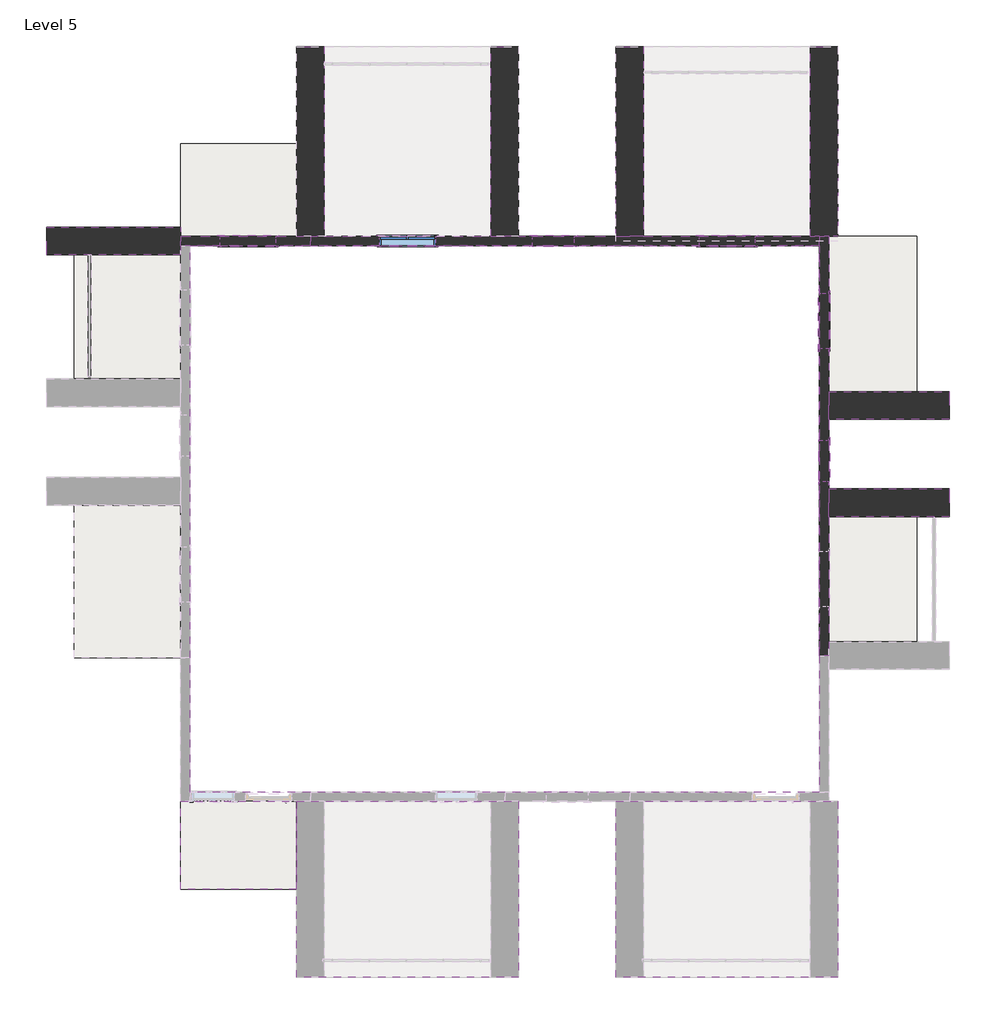
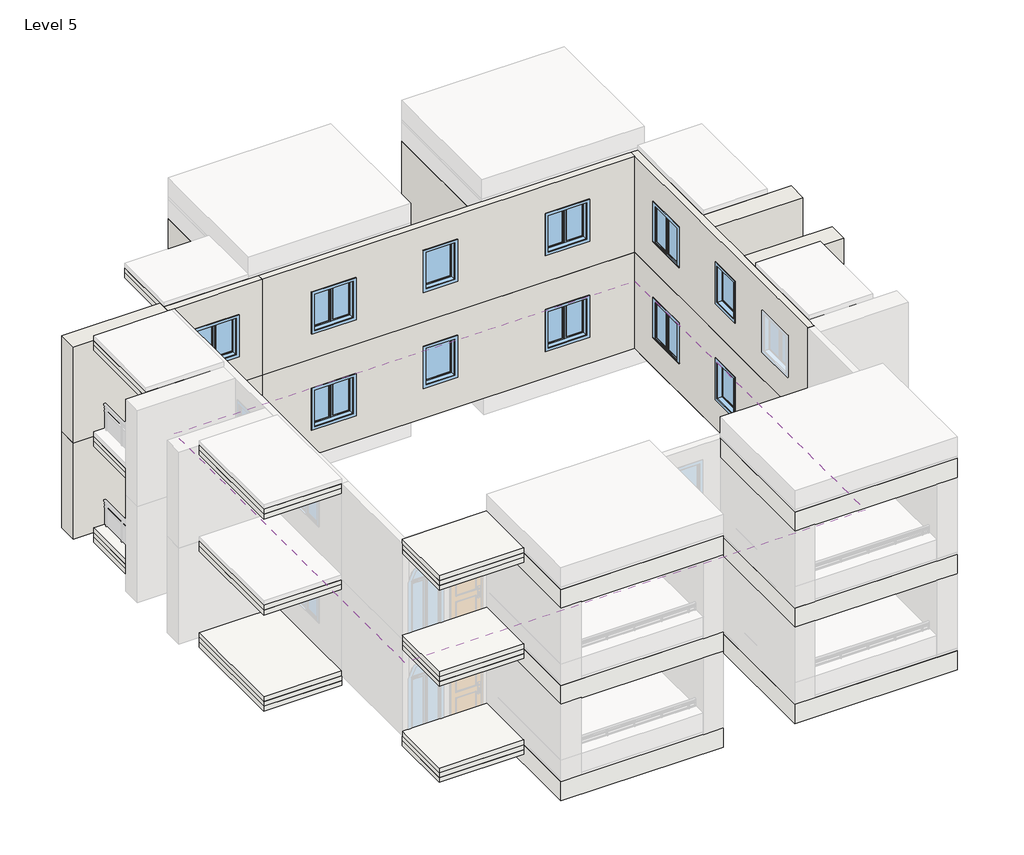
# One storey, part 2 of 4: 20 walls, 16 slabs, 12 windows, 1 covering.
# Revit data of these elements (continued)
# Materials (continued)
#   "Damp-proofing": class "Generic", colour RGB 127 127 127, transparency 0, Description = "Damp-proofing", Cost = 0
#   "Concrete Masonry Units": class "Masonry", colour RGB 227 227 227, transparency 0, Description = "Concrete masonry units", Cost = 0
#   "Door - Frame": colour RGB 118 70 51, transparency 0, Cost = 0
#   "Glass": class "Glass", colour RGB 0 128 192, transparency 0.75, Description = "Soda Lime Glass", Cost = 0
#   "Sash": class "Wood", colour RGB 224 178 126, transparency 0
#   "Trim": class "Wood", colour RGB 224 178 126, transparency 0
#   "Gypsum Wall Board": class "Generic", colour RGB 127 127 127, transparency 0, Description = "Gypsum Wall Board", Cost = 0
#   "Default Wall": colour RGB 128 128 128, transparency 0
#   "Tile, Porcelain, 4in": class "Generic", colour RGB 89 87 158, transparency 0, Description = "Porcelain tile, 4\", white", Cost = 0
#   "Parking Stripe": class "Paint", colour RGB 250 250 91, transparency 0, Cost = 0
